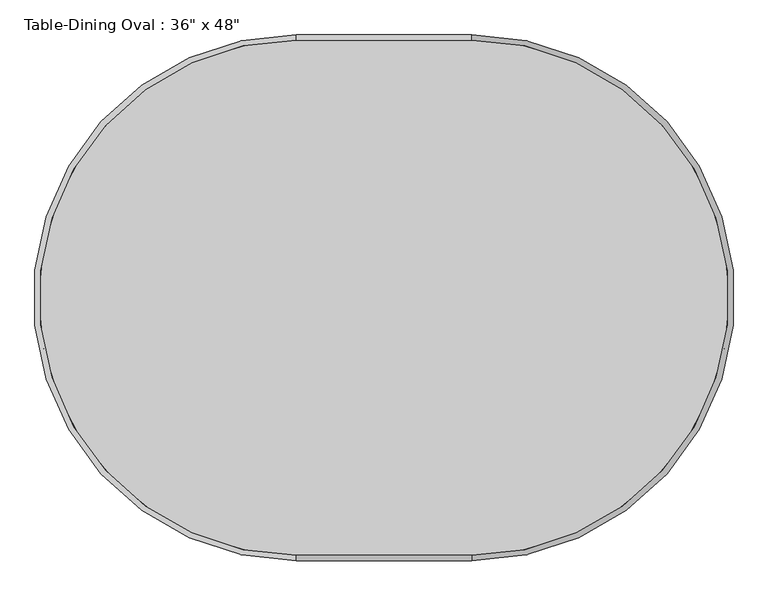
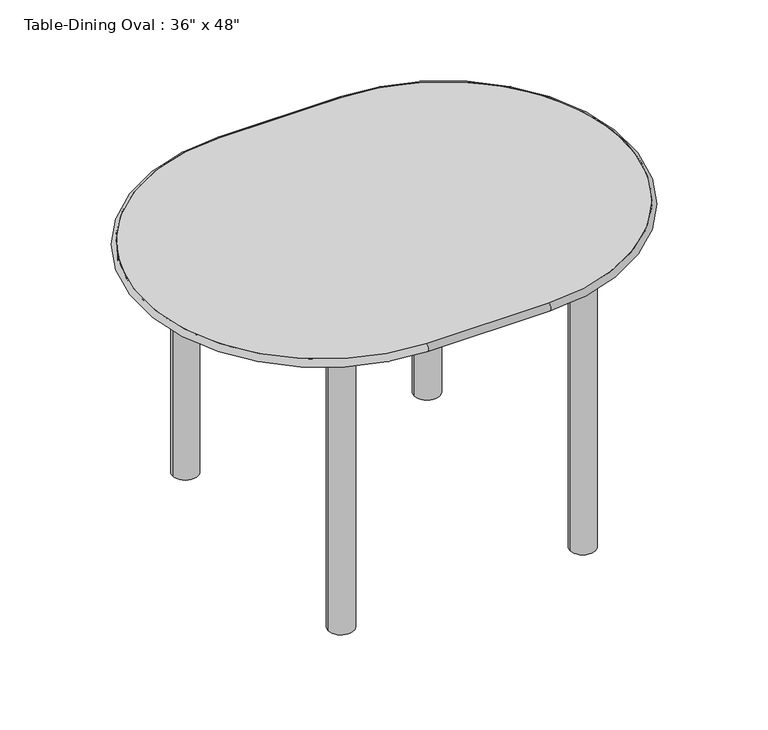
"""IFC4 building model written with IfcOpenShell, lengths in millimetres: furniture geometry."""

from ifc_helpers import new_model, si_unit, point, frame, frame_2d, origin, origin_with_axes, place, context, project, spatial, polyline, circle_curve, ellipse_curve, trimmed, segment, composite_curve, outline, extrude, source, transform, mapped, element, save
from ifc_brep_helpers import plane_surface, cylinder_surface, revolved_surface, advanced_brep


def furniture_be1c6672(model_context):
    return source(origin(), model_context, "Body", "SolidModel", [
        advanced_brep(
        [(-554.2196721, -805.7733607, 762.0), (-554.2196721, -805.7733607, 742.95), (-249.4196721, -805.7733607, 742.95), (-249.4196721, -805.7733607, 762.0), (-249.4196721, 89.5766393, 762.0), (-249.4196721, 89.5766393, 742.95), (-554.2196721, 89.5766393, 742.95), (-554.2196721, 89.5766393, 762.0)],
        [
            (0, 1, circle_curve(frame((-554.2196721, -805.7733607, 752.475), z_axis=(1.0, 0.0, 0.0), x_axis=(0.0, 1.0, 0.0)), 9.525)),
            (1, 2),
            (2, 3, circle_curve(frame((-249.4196721, -805.7733607, 752.475), z_axis=(-1.0, 0.0, 0.0), x_axis=(0.0, 1.0, 0.0)), 9.525)),
            (3, 0),
            (1, 0),
            (3, 2),
            (4, 3, circle_curve(frame((-249.4196721, -358.0983607, 762.0), z_axis=(0.0, 0.0, -1.0), x_axis=(0.0, -1.0, 0.0)), 447.675)),
            (2, 5, circle_curve(frame((-249.4196721, -358.0983607, 742.95), z_axis=(0.0, 0.0, 1.0), x_axis=(0.0, -1.0, 0.0)), 447.675)),
            (5, 4, circle_curve(frame((-249.4196721, 89.5766393, 752.475), z_axis=(1.0, 0.0, 0.0), x_axis=(0.0, -1.0, 0.0)), 9.525)),
            (4, 5),
            (5, 6),
            (6, 7, circle_curve(frame((-554.2196721, 89.5766393, 752.475), z_axis=(1.0, 0.0, 0.0), x_axis=(0.0, -1.0, 0.0)), 9.525)),
            (7, 4),
            (7, 6),
            (0, 7, circle_curve(frame((-554.2196721, -358.0983607, 762.0), z_axis=(0.0, 0.0, -1.0), x_axis=(0.0, 1.0, 0.0)), 447.675)),
            (6, 1, circle_curve(frame((-554.2196721, -358.0983607, 742.95), z_axis=(0.0, 0.0, 1.0), x_axis=(0.0, 1.0, 0.0)), 447.675)),
        ],
        [
            cylinder_surface(frame((-554.2196721, -805.7733607, 752.475), z_axis=(-1.0, 0.0, 0.0), x_axis=(0.0, 1.0, 0.0)), 9.525),
            plane_surface(frame((-554.2196721, -805.7733607, 762.0), z_axis=(0.0, 1.0, 0.0), x_axis=(1.0, 0.0, 0.0))),
            revolved_surface(trimmed(ellipse_curve(frame((-249.4196721, -805.7733607, 752.475), z_axis=(-1.0, 0.0, 0.0), x_axis=(0.0, 1.0, 0.0)), 9.525, 9.525), [point((-249.4196721, -805.7733607, 742.95))], [point((-249.4196721, -805.7733607, 762.0))], True, "CARTESIAN"), (-249.4196721, -358.0983607, 0.0), (0.0, 0.0, 1.0)),
            revolved_surface(polyline([(-249.4196721, -805.7733607, 762.0), (-249.4196721, -805.7733607, 742.95)]), (-249.4196721, -358.0983607, 0.0), (0.0, 0.0, 1.0)),
            cylinder_surface(frame((-249.4196721, 89.5766393, 752.475), z_axis=(1.0, 0.0, 0.0), x_axis=(0.0, -1.0, 0.0)), 9.525),
            plane_surface(frame((-249.4196721, 89.5766393, 762.0), z_axis=(0.0, -1.0, 0.0), x_axis=(-1.0, 0.0, 0.0))),
            revolved_surface(trimmed(ellipse_curve(frame((-554.2196721, 89.5766393, 752.475), z_axis=(1.0, 0.0, 0.0), x_axis=(0.0, -1.0, 0.0)), 9.525, 9.525), [point((-554.2196721, 89.5766393, 742.95))], [point((-554.2196721, 89.5766393, 762.0))], True, "CARTESIAN"), (-554.2196721, -358.0983607, 0.0), (0.0, 0.0, 1.0)),
            revolved_surface(polyline([(-554.2196721, 89.57663930000001, 762.0), (-554.2196721, 89.57663930000001, 742.95)]), (-554.2196721, -358.0983607, 0.0), (0.0, 0.0, 1.0)),
        ],
        [
            (0, [[1, 2, 3, 4]]),
            (1, [[5, -4, 6, -2]]),
            (2, [[7, -3, 8, 9]]),
            (3, [[-8, -6, -7, 10]]),
            (4, [[-9, 11, 12, 13]]),
            (5, [[-10, -13, 14, -11]]),
            (6, [[15, -12, 16, -1]]),
            (7, [[-16, -14, -15, -5]]),
        ],
    ),
        extrude(outline(composite_curve([segment(trimmed(circle_curve(frame_2d((-703.4446721, -21.5483607)), 31.75), [point((-735.1946721, -21.5483607))], [point((-671.6946721, -21.5483607))], False, "CARTESIAN"), True, "CONTINUOUS"), segment(trimmed(circle_curve(frame_2d((-703.4446721, -21.5483607)), 31.75), [point((-671.6946721, -21.5483607))], [point((-735.1946721, -21.5483607))], False, "CARTESIAN"), True, "CONTINUOUS")], self_intersect=False)), origin_with_axes(), (0.0, 0.0, 1.0), 742.95),
        extrude(outline(composite_curve([segment(trimmed(circle_curve(frame_2d((-703.4446721, -694.6483607)), 31.75), [point((-735.1946721, -694.6483607))], [point((-671.6946721, -694.6483607))], False, "CARTESIAN"), True, "CONTINUOUS"), segment(trimmed(circle_curve(frame_2d((-703.4446721, -694.6483607)), 31.75), [point((-671.6946721, -694.6483607))], [point((-735.1946721, -694.6483607))], False, "CARTESIAN"), True, "CONTINUOUS")], self_intersect=False)), origin_with_axes(), (0.0, 0.0, 1.0), 742.95),
        extrude(outline(composite_curve([segment(trimmed(circle_curve(frame_2d((-100.1946721, -21.5483607)), 31.75), [point((-131.9446721, -21.5483607))], [point((-68.4446721, -21.5483607))], False, "CARTESIAN"), True, "CONTINUOUS"), segment(trimmed(circle_curve(frame_2d((-100.1946721, -21.5483607)), 31.75), [point((-68.4446721, -21.5483607))], [point((-131.9446721, -21.5483607))], False, "CARTESIAN"), True, "CONTINUOUS")], self_intersect=False)), origin_with_axes(), (0.0, 0.0, 1.0), 742.95),
        extrude(outline(composite_curve([segment(trimmed(circle_curve(frame_2d((-100.1946721, -694.6483607)), 31.75), [point((-131.9446721, -694.6483607))], [point((-68.4446721, -694.6483607))], False, "CARTESIAN"), True, "CONTINUOUS"), segment(trimmed(circle_curve(frame_2d((-100.1946721, -694.6483607)), 31.75), [point((-68.4446721, -694.6483607))], [point((-131.9446721, -694.6483607))], False, "CARTESIAN"), True, "CONTINUOUS")], self_intersect=False)), origin_with_axes(), (0.0, 0.0, 1.0), 742.95),
        extrude(outline(polyline([(-81.1446721, -2.4983607), (-81.1446721, -713.6983607), (-722.4946721, -713.6983607), (-722.4946721, -2.4983607), (-81.1446721, -2.4983607)]), holes=[polyline([(-100.1946721, -21.5483607), (-703.4446721, -21.5483607), (-703.4446721, -694.6483607), (-100.1946721, -694.6483607), (-100.1946721, -21.5483607)])]), frame((0.0, 0.0, 692.15), z_axis=(0.0, 0.0, 1.0), x_axis=(1.0, 0.0, 0.0)), (0.0, 0.0, 1.0), 50.8),
        extrude(outline(composite_curve([segment(polyline([(-554.2196721, 89.5766393), (-249.4196721, 89.5766393)]), True, "CONTINUOUS"), segment(trimmed(circle_curve(frame_2d((-249.4196721, -358.0983607)), 447.675), [point((-249.4196721, 89.5766393))], [point((198.2553279, -358.0983607))], False, "CARTESIAN"), True, "CONTINUOUS"), segment(trimmed(circle_curve(frame_2d((-249.4196721, -358.0983607)), 447.675), [point((198.2553279, -358.0983607))], [point((-249.4196721, -805.7733607))], False, "CARTESIAN"), True, "CONTINUOUS"), segment(polyline([(-249.4196721, -805.7733607), (-554.2196721, -805.7733607)]), True, "CONTINUOUS"), segment(trimmed(circle_curve(frame_2d((-554.2196721, -358.0983607)), 447.675), [point((-554.2196721, -805.7733607))], [point((-1001.8946721, -358.0983607))], False, "CARTESIAN"), True, "CONTINUOUS"), segment(trimmed(circle_curve(frame_2d((-554.2196721, -358.0983607)), 447.675), [point((-1001.8946721, -358.0983607))], [point((-554.2196721, 89.5766393))], False, "CARTESIAN"), True, "CONTINUOUS")], self_intersect=False)), frame((0.0, 0.0, 742.95), z_axis=(0.0, 0.0, 1.0), x_axis=(1.0, 0.0, 0.0)), (0.0, 0.0, 1.0), 19.05),
    ])


if __name__ == "__main__":
    model = new_model("IFC4")
    model_context = context("Model", 3, world=origin())
    ifc_project = project(units=[si_unit("LENGTHUNIT", "METRE", prefix="MILLI")], contexts=[model_context])
    site = spatial("IfcSite", under=ifc_project)
    building = spatial("IfcBuilding", under=site)
    placement = place(None, origin())
    furniture_shape = furniture_be1c6672(model_context)
    element("IfcFurniture", 1, ObjectType="Table-Dining Oval : 36\" x 48\"", at=placement, inside=building, context=model_context, shape_type="MappedRepresentation", body=[
        mapped(furniture_shape, transform((0.0, 0.0, 0.0), x_axis=(1.0, 0.0, 0.0), y_axis=(0.0, 1.0, 0.0), z_axis=(0.0, 0.0, 1.0))),
    ])
    save(model, "model.ifc")

# Revit data of these elements
# Type "Table-Dining Oval : 36\" x 48\""
#   Assembly Code = "E2020200"
#   Length = 4' - 0"
#   Width = 3' - 0"
#   Base Material = Steel, Chrome Plated
#   Top Material = Glass
#   Default Elevation = 0
#   Description = (empty or 0)
# Element 1 (IfcFurniture, "Table-Dining Oval : 36\" x 48\"")
#   Materials on its faces: "Steel, Chrome Plated", "Glass - Clear, Grey", "Glass"
# Materials
#   "Steel, Chrome Plated": class "Metal", colour RGB 17 17 17, transparency 0, Description = "Chromiuim plated steel", Cost = 0
#   "Glass": class "Glass", colour RGB 0 128 192, transparency 0.75, Description = "Soda Lime Glass", Cost = 0
#   "Glass - Clear, Grey": class "Glass", colour RGB 252 255 255, transparency 0.64
